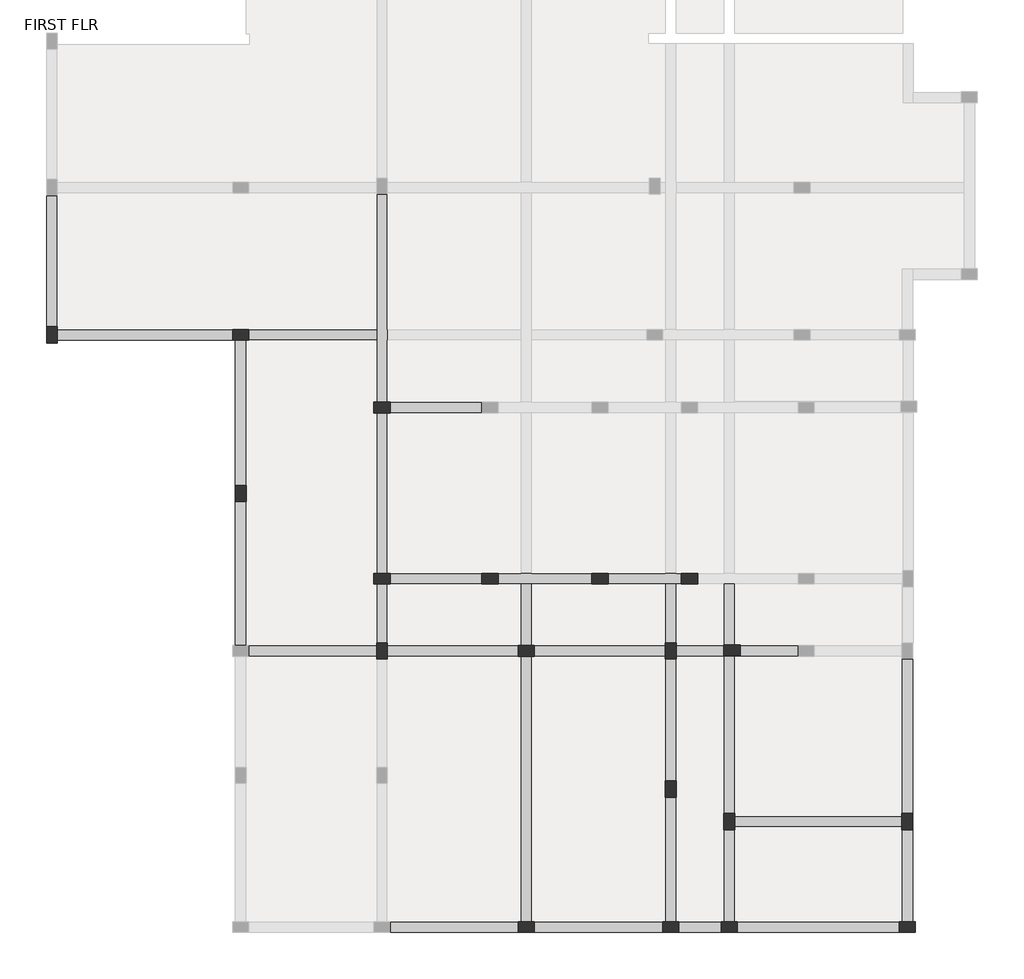
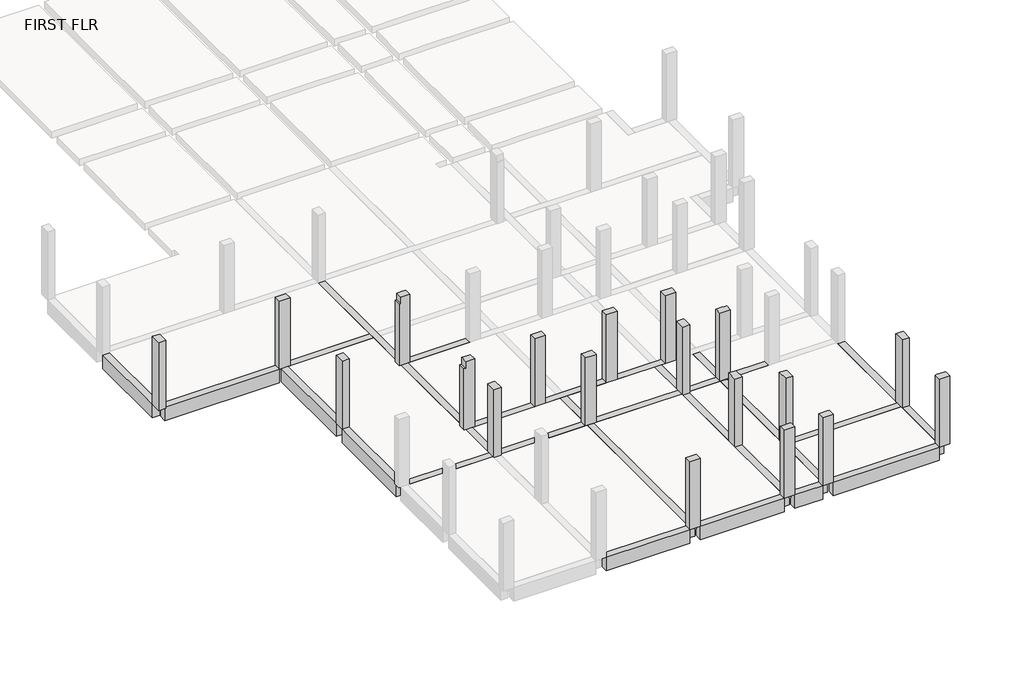
# One storey, part 2 of 5: 31 beams, 19 columns.
"""IFC4 building model written with IfcOpenShell, lengths in millimetres."""

from ifc_helpers import new_model, si_unit, frame, origin, place, context, project, spatial, polyline, outline, extrude, faceted_brep, element, save

model = new_model("IFC4")

# Units and contexts
model_context = context("Model", 3, world=origin())
ifc_project = project(units=[si_unit("LENGTHUNIT", "METRE", prefix="MILLI")], contexts=[model_context])

# Site, building, storey
site = spatial("IfcSite", under=ifc_project)
building = spatial("IfcBuilding", under=site)
storey = spatial("IfcBuildingStorey", under=building, Name="FIRST FLR", Elevation=3000.0)

# Beams
placement = place(None, origin())
element("IfcBeam", 1, ObjectType="M_Concrete-Rectangular Beam : 300 x 600mm", at=placement, inside=storey, context=model_context, shape_type="SweptSolid", body=[
    extrude(outline(polyline([(-10828.8105653, -2764.4535766), (-11128.8105653, -2764.4535766), (-11128.8105653, 876.1713929), (-10828.8105653, 876.1713929), (-10828.8105653, -2764.4535766)])), frame((0.0, 0.0, 2400.0), z_axis=(0.0, 0.0, 1.0), x_axis=(1.0, 0.0, 0.0)), (0.0, 0.0, 1.0), 600.0),
])
element("IfcBeam", 2, ObjectType="M_Concrete-Rectangular Beam : 300 x 600mm", at=placement, inside=storey, context=model_context, shape_type="Brep", body=[
    faceted_brep([(-5963.8105653, -3139.4535766, 3000.0), (-5963.8105653, -2839.4535766, 3000.0), (-10828.8105653, -2839.4535766, 3000.0), (-10828.8105653, -3139.4535766, 3000.0), (-5963.8105653, -3139.4535766, 2400.0), (-10828.8105653, -3139.4535766, 2400.0), (-5963.8105653, -2839.4535766, 2400.0), (-10828.8105653, -2839.4535766, 2400.0), (-5963.8105653, -2839.4535766, 2700.0), (-10828.8105653, -2839.4535766, 2700.0)], [[[0, 1, 2, 3]], [[4, 0, 3, 5]], [[6, 4, 5, 7]], [[2, 1, 8, 6, 7, 9]], [[1, 0, 4, 6, 8]], [[3, 2, 9, 7, 5]]]),
])
element("IfcBeam", 3, ObjectType="M_Concrete-Rectangular Beam : 300 x 600mm", at=placement, inside=storey, context=model_context, shape_type="Brep", body=[
    faceted_brep([(-5588.8105653, -7169.0760584, 3000.0), (-5588.8105653, -3139.4535766, 3000.0), (-5888.8105653, -3139.4535766, 3000.0), (-5888.8105653, -7169.0760584, 3000.0), (-5888.8105653, -3139.4535766, 2400.0), (-5888.8105653, -7169.0760584, 2400.0), (-5588.8105653, -3139.4535766, 2400.0), (-5588.8105653, -7169.0760584, 2400.0), (-5588.8105653, -7169.0760584, 2700.0), (-5588.8105653, -3139.4535766, 2700.0)], [[[0, 1, 2, 3]], [[3, 2, 4, 5]], [[5, 4, 6, 7]], [[1, 0, 8, 7, 6, 9]], [[6, 4, 2, 1, 9]], [[0, 3, 5, 7, 8]]]),
])
element("IfcBeam", 4, ObjectType="M_Concrete-Rectangular Beam : 300 x 600mm", at=placement, inside=storey, context=model_context, shape_type="Brep", body=[
    faceted_brep([(-5588.8105653, -11607.8970059, 3000.0), (-5588.8105653, -7619.0760584, 3000.0), (-5888.8105653, -7619.0760584, 3000.0), (-5888.8105653, -11607.8970059, 3000.0), (-5888.8105653, -7619.0760584, 2400.0), (-5888.8105653, -11607.8970059, 2400.0), (-5588.8105653, -7619.0760584, 2400.0), (-5588.8105653, -11607.8970059, 2400.0), (-5588.8105653, -11607.8970059, 2700.0), (-5588.8105653, -7619.0760584, 2700.0)], [[[0, 1, 2, 3]], [[3, 2, 4, 5]], [[5, 4, 6, 7]], [[1, 0, 8, 7, 6, 9]], [[0, 3, 5, 7, 8]], [[6, 4, 2, 1, 9]]]),
])
element("IfcBeam", 5, ObjectType="M_Concrete-Rectangular Beam : 300 x 600mm", at=placement, inside=storey, context=model_context, shape_type="SweptSolid", body=[
    extrude(outline(polyline([(1949.7296816, -19272.5304373), (1949.7296816, -19572.5304373), (-1596.7865686, -19572.5304373), (-1596.7865686, -19272.5304373), (1949.7296816, -19272.5304373)])), frame((0.0, 0.0, 2400.0), z_axis=(0.0, 0.0, 1.0), x_axis=(1.0, 0.0, 0.0)), (0.0, 0.0, 1.0), 600.0),
])
element("IfcBeam", 6, ObjectType="M_Concrete-Rectangular Beam : 300 x 600mm", at=placement, inside=storey, context=model_context, shape_type="SweptSolid", body=[
    extrude(outline(polyline([(5957.5248054, -19272.5304373), (5957.5248054, -19572.5304373), (2399.7296816, -19572.5304373), (2399.7296816, -19272.5304373), (5957.5248054, -19272.5304373)])), frame((0.0, 0.0, 2400.0), z_axis=(0.0, 0.0, 1.0), x_axis=(1.0, 0.0, 0.0)), (0.0, 0.0, 1.0), 600.0),
])
element("IfcBeam", 7, ObjectType="M_Concrete-Rectangular Beam : 300 x 600mm", at=placement, inside=storey, context=model_context, shape_type="SweptSolid", body=[
    extrude(outline(polyline([(7581.8679014, -19272.5304373), (7581.8679014, -19572.5304373), (6407.5248054, -19572.5304373), (6407.5248054, -19272.5304373), (7581.8679014, -19272.5304373)])), frame((0.0, 0.0, 2400.0), z_axis=(0.0, 0.0, 1.0), x_axis=(1.0, 0.0, 0.0)), (0.0, 0.0, 1.0), 600.0),
])
element("IfcBeam", 8, ObjectType="M_Concrete-Rectangular Beam : 300 x 600mm", at=placement, inside=storey, context=model_context, shape_type="SweptSolid", body=[
    extrude(outline(polyline([(12524.1163908, -19272.5304373), (12524.1163908, -19572.5304373), (8031.8679014, -19572.5304373), (8031.8679014, -19272.5304373), (12524.1163908, -19272.5304373)])), frame((0.0, 0.0, 2400.0), z_axis=(0.0, 0.0, 1.0), x_axis=(1.0, 0.0, 0.0)), (0.0, 0.0, 1.0), 600.0),
])
element("IfcBeam", 9, ObjectType="M_Concrete-Rectangular Beam : 300 x 600mm", at=placement, inside=storey, context=model_context, shape_type="Brep", body=[
    faceted_brep([(12599.1163908, -19272.5304373, 3000.0), (12899.1163908, -19272.5304373, 3000.0), (12899.1163908, -16719.1579597, 3000.0), (12599.1163908, -16719.1579597, 3000.0), (12899.1163908, -19272.5304373, 2400.0), (12899.1163908, -16719.1579597, 2400.0), (12599.1163908, -19272.5304373, 2400.0), (12599.1163908, -16719.1579597, 2400.0), (12599.1163908, -16719.1579597, 2700.0), (12599.1163908, -19272.5304373, 2700.0)], [[[0, 1, 2, 3]], [[1, 4, 5, 2]], [[4, 6, 7, 5]], [[0, 3, 8, 7, 6, 9]], [[6, 4, 1, 0, 9]], [[3, 2, 5, 7, 8]]]),
])
element("IfcBeam", 10, ObjectType="M_Concrete-Rectangular Beam : 300 x 600mm", at=placement, inside=storey, context=model_context, shape_type="Brep", body=[
    faceted_brep([(12599.1163908, -16269.1579597, 3000.0), (12899.1163908, -16269.1579597, 3000.0), (12899.1163908, -11982.8970059, 3000.0), (12599.1163908, -11982.8970059, 3000.0), (12899.1163908, -16269.1579597, 2400.0), (12899.1163908, -11982.8970059, 2400.0), (12599.1163908, -16269.1579597, 2400.0), (12599.1163908, -11982.8970059, 2400.0), (12599.1163908, -11982.8970059, 2700.0), (12599.1163908, -16269.1579597, 2700.0)], [[[0, 1, 2, 3]], [[1, 4, 5, 2]], [[4, 6, 7, 5]], [[0, 3, 8, 7, 6, 9]], [[6, 4, 1, 0, 9]], [[3, 2, 5, 7, 8]]]),
])
element("IfcBeam", 11, ObjectType="M_Concrete-Rectangular Beam : 300 x 600mm", at=placement, inside=storey, context=model_context, shape_type="Brep", body=[
    faceted_brep([(-1971.7865686, -9907.1078267, 3000.0), (-1971.7865686, -11532.8970059, 3000.0), (-1671.7865686, -11532.8970059, 3000.0), (-1671.7865686, -9907.1078267, 3000.0), (-1671.7865686, -11532.8970059, 2700.0), (-1671.7865686, -11532.8970059, 2400.0), (-1671.7865686, -9907.1078267, 2400.0), (-1671.7865686, -9907.1078267, 2700.0), (-1971.7865686, -11532.8970059, 2400.0), (-1971.7865686, -9907.1078267, 2400.0), (-1971.7865686, -9907.1078267, 2700.0), (-1971.7865686, -11532.8970059, 2700.0)], [[[0, 1, 2, 3]], [[3, 2, 4, 5, 6, 7]], [[6, 5, 8, 9]], [[1, 0, 10, 9, 8, 11]], [[0, 3, 7, 6, 9, 10]], [[8, 5, 4, 2, 1, 11]]]),
])
element("IfcBeam", 12, ObjectType="M_Concrete-Rectangular Beam : 300 x 600mm", at=placement, inside=storey, context=model_context, shape_type="Brep", body=[
    faceted_brep([(-1671.7865686, 916.1713929, 3000.0), (-1971.7865686, 916.1713929, 3000.0), (-1971.7865686, -2839.4535766, 3000.0), (-1971.7865686, -3139.4535766, 3000.0), (-1971.7865686, -4851.6229916, 3000.0), (-1671.7865686, -4851.6229916, 3000.0), (-1671.7865686, -3139.4535766, 3000.0), (-1671.7865686, -2839.4535766, 3000.0), (-1971.7865686, 916.1713929, 2400.0), (-1971.7865686, -2839.4535766, 2400.0), (-1971.7865686, -3139.4535766, 2400.0), (-1971.7865686, -4851.6229916, 2400.0), (-1971.7865686, -4851.6229916, 2700.0), (-1971.7865686, 916.1713929, 2700.0), (-1671.7865686, 916.1713929, 2400.0), (-1671.7865686, -2839.4535766, 2400.0), (-1671.7865686, -3139.4535766, 2400.0), (-1671.7865686, -4851.6229916, 2400.0), (-1671.7865686, 916.1713929, 2700.0), (-1671.7865686, -4851.6229916, 2700.0)], [[[0, 1, 2, 3, 4, 5, 6, 7]], [[8, 9, 10, 11, 12, 4, 3, 2, 1, 13]], [[8, 14, 15, 16, 17, 11, 10, 9]], [[17, 16, 15, 14, 18, 0, 7, 6, 5, 19]], [[1, 0, 18, 14, 8, 13]], [[5, 4, 12, 11, 17, 19]]]),
])
element("IfcBeam", 13, ObjectType="M_Concrete-Rectangular Beam : 300 x 600mm", at=placement, inside=storey, context=model_context, shape_type="Brep", body=[
    faceted_brep([(-1671.7865686, -5151.6229916, 3000.0), (-1971.7865686, -5151.6229916, 3000.0), (-1971.7865686, -9607.1078267, 3000.0), (-1671.7865686, -9607.1078267, 3000.0), (-1971.7865686, -5151.6229916, 2700.0), (-1971.7865686, -5151.6229916, 2400.0), (-1971.7865686, -9607.1078267, 2400.0), (-1971.7865686, -9607.1078267, 2700.0), (-1671.7865686, -5151.6229916, 2400.0), (-1671.7865686, -9607.1078267, 2400.0), (-1671.7865686, -9607.1078267, 2700.0), (-1671.7865686, -5151.6229916, 2700.0)], [[[0, 1, 2, 3]], [[2, 1, 4, 5, 6, 7]], [[5, 8, 9, 6]], [[0, 3, 10, 9, 8, 11]], [[1, 0, 11, 8, 5, 4]], [[3, 2, 7, 6, 9, 10]]]),
])
element("IfcBeam", 14, ObjectType="M_Concrete-Rectangular Beam : 300 x 600mm", at=placement, inside=storey, context=model_context, shape_type="Brep", body=[
    faceted_brep([(2324.7296816, -11907.8970059, 3000.0), (2024.7296816, -11907.8970059, 3000.0), (2024.7296816, -19272.5304373, 3000.0), (2324.7296816, -19272.5304373, 3000.0), (2024.7296816, -11907.8970059, 2700.0), (2024.7296816, -11907.8970059, 2400.0), (2024.7296816, -19272.5304373, 2400.0), (2024.7296816, -19272.5304373, 2700.0), (2324.7296816, -11907.8970059, 2400.0), (2324.7296816, -19272.5304373, 2400.0), (2324.7296816, -19272.5304373, 2700.0), (2324.7296816, -11907.8970059, 2700.0)], [[[0, 1, 2, 3]], [[2, 1, 4, 5, 6, 7]], [[5, 8, 9, 6]], [[0, 3, 10, 9, 8, 11]], [[1, 0, 11, 8, 5, 4]], [[3, 2, 7, 6, 9, 10]]]),
])
element("IfcBeam", 15, ObjectType="M_Concrete-Rectangular Beam : 300 x 600mm", at=placement, inside=storey, context=model_context, shape_type="Brep", body=[
    faceted_brep([(6332.5248054, -11982.8970059, 3000.0), (6032.5248054, -11982.8970059, 3000.0), (6032.5248054, -15369.1579597, 3000.0), (6332.5248054, -15369.1579597, 3000.0), (6032.5248054, -11982.8970059, 2700.0), (6032.5248054, -11982.8970059, 2400.0), (6032.5248054, -15369.1579597, 2400.0), (6032.5248054, -15369.1579597, 2700.0), (6332.5248054, -11982.8970059, 2400.0), (6332.5248054, -15369.1579597, 2400.0), (6332.5248054, -15369.1579597, 2700.0), (6332.5248054, -11982.8970059, 2700.0)], [[[0, 1, 2, 3]], [[2, 1, 4, 5, 6, 7]], [[5, 8, 9, 6]], [[0, 3, 10, 9, 8, 11]], [[1, 0, 11, 8, 5, 4]], [[3, 2, 7, 6, 9, 10]]]),
])
element("IfcBeam", 16, ObjectType="M_Concrete-Rectangular Beam : 300 x 600mm", at=placement, inside=storey, context=model_context, shape_type="Brep", body=[
    faceted_brep([(6032.5248054, -19272.5304373, 3000.0), (6332.5248054, -19272.5304373, 3000.0), (6332.5248054, -15819.1579597, 3000.0), (6032.5248054, -15819.1579597, 3000.0), (6032.5248054, -15819.1579597, 2700.0), (6032.5248054, -15819.1579597, 2400.0), (6032.5248054, -19272.5304373, 2400.0), (6032.5248054, -19272.5304373, 2700.0), (6332.5248054, -19272.5304373, 2400.0), (6332.5248054, -15819.1579597, 2400.0), (6332.5248054, -19272.5304373, 2700.0), (6332.5248054, -15819.1579597, 2700.0)], [[[0, 1, 2, 3]], [[0, 3, 4, 5, 6, 7]], [[8, 6, 5, 9]], [[2, 1, 10, 8, 9, 11]], [[1, 0, 7, 6, 8, 10]], [[3, 2, 11, 9, 5, 4]]]),
])
element("IfcBeam", 17, ObjectType="M_Concrete-Rectangular Beam : 300 x 600mm", at=placement, inside=storey, context=model_context, shape_type="Brep", body=[
    faceted_brep([(7656.8679014, -19272.5304373, 3000.0), (7956.8679014, -19272.5304373, 3000.0), (7956.8679014, -16719.1579597, 3000.0), (7656.8679014, -16719.1579597, 3000.0), (7656.8679014, -16719.1579597, 2700.0), (7656.8679014, -16719.1579597, 2400.0), (7656.8679014, -19272.5304373, 2400.0), (7656.8679014, -19272.5304373, 2700.0), (7956.8679014, -19272.5304373, 2400.0), (7956.8679014, -16719.1579597, 2400.0), (7956.8679014, -19272.5304373, 2700.0), (7956.8679014, -16719.1579597, 2700.0)], [[[0, 1, 2, 3]], [[0, 3, 4, 5, 6, 7]], [[8, 6, 5, 9]], [[2, 1, 10, 8, 9, 11]], [[1, 0, 7, 6, 8, 10]], [[3, 2, 11, 9, 5, 4]]]),
])
element("IfcBeam", 18, ObjectType="M_Concrete-Rectangular Beam : 300 x 600mm", at=placement, inside=storey, context=model_context, shape_type="Brep", body=[
    faceted_brep([(-5513.8105653, -2839.4535766, 3000.0), (-5513.8105653, -3139.4535766, 3000.0), (-1971.7865686, -3139.4535766, 3000.0), (-1971.7865686, -2839.4535766, 3000.0), (-5513.8105653, -3139.4535766, 2700.0), (-5513.8105653, -3139.4535766, 2400.0), (-1971.7865686, -3139.4535766, 2400.0), (-1971.7865686, -3139.4535766, 2700.0), (-5513.8105653, -2839.4535766, 2400.0), (-1971.7865686, -2839.4535766, 2400.0), (-1971.7865686, -2839.4535766, 2700.0), (-5513.8105653, -2839.4535766, 2700.0)], [[[0, 1, 2, 3]], [[2, 1, 4, 5, 6, 7]], [[5, 8, 9, 6]], [[0, 3, 10, 9, 8, 11]], [[1, 0, 11, 8, 5, 4]], [[3, 2, 7, 6, 9, 10]]]),
])
element("IfcBeam", 19, ObjectType="M_Concrete-Rectangular Beam : 300 x 600mm", at=placement, inside=storey, context=model_context, shape_type="Brep", body=[
    faceted_brep([(-1596.7865686, -4851.6229916, 3000.0), (-1596.7865686, -5151.6229916, 3000.0), (949.7296816, -5151.6229916, 3000.0), (949.7296816, -4851.6229916, 3000.0), (-1596.7865686, -5151.6229916, 2700.0), (-1596.7865686, -5151.6229916, 2400.0), (949.7296816, -5151.6229916, 2400.0), (949.7296816, -5151.6229916, 2700.0), (-1596.7865686, -4851.6229916, 2400.0), (949.7296816, -4851.6229916, 2400.0), (949.7296816, -4851.6229916, 2700.0), (-1596.7865686, -4851.6229916, 2700.0)], [[[0, 1, 2, 3]], [[2, 1, 4, 5, 6, 7]], [[5, 8, 9, 6]], [[0, 3, 10, 9, 8, 11]], [[1, 0, 11, 8, 5, 4]], [[3, 2, 7, 6, 9, 10]]]),
])
element("IfcBeam", 20, ObjectType="M_Concrete-Rectangular Beam : 300 x 600mm", at=placement, inside=storey, context=model_context, shape_type="Brep", body=[
    faceted_brep([(-1971.7865686, -11907.8970059, 3000.0), (-1971.7865686, -11607.8970059, 3000.0), (-5513.8105653, -11607.8970059, 3000.0), (-5513.8105653, -11907.8970059, 3000.0), (-5513.8105653, -11907.8970059, 2700.0), (-5513.8105653, -11907.8970059, 2400.0), (-1971.7865686, -11907.8970059, 2400.0), (-1971.7865686, -11907.8970059, 2700.0), (-1971.7865686, -11607.8970059, 2400.0), (-5513.8105653, -11607.8970059, 2400.0), (-1971.7865686, -11607.8970059, 2700.0), (-5513.8105653, -11607.8970059, 2700.0)], [[[0, 1, 2, 3]], [[0, 3, 4, 5, 6, 7]], [[8, 6, 5, 9]], [[2, 1, 10, 8, 9, 11]], [[1, 0, 7, 6, 8, 10]], [[3, 2, 11, 9, 5, 4]]]),
])
element("IfcBeam", 21, ObjectType="M_Concrete-Rectangular Beam : 300 x 600mm", at=placement, inside=storey, context=model_context, shape_type="Brep", body=[
    faceted_brep([(1949.7296816, -11907.8970059, 3000.0), (1949.7296816, -11607.8970059, 3000.0), (-1671.7865686, -11607.8970059, 3000.0), (-1671.7865686, -11907.8970059, 3000.0), (-1671.7865686, -11907.8970059, 2700.0), (-1671.7865686, -11907.8970059, 2400.0), (1949.7296816, -11907.8970059, 2400.0), (1949.7296816, -11907.8970059, 2700.0), (1949.7296816, -11607.8970059, 2400.0), (-1671.7865686, -11607.8970059, 2400.0), (1949.7296816, -11607.8970059, 2700.0), (-1671.7865686, -11607.8970059, 2700.0)], [[[0, 1, 2, 3]], [[0, 3, 4, 5, 6, 7]], [[8, 6, 5, 9]], [[2, 1, 10, 8, 9, 11]], [[1, 0, 7, 6, 8, 10]], [[3, 2, 11, 9, 5, 4]]]),
])
element("IfcBeam", 22, ObjectType="M_Concrete-Rectangular Beam : 300 x 600mm", at=placement, inside=storey, context=model_context, shape_type="Brep", body=[
    faceted_brep([(6032.5248054, -11907.8970059, 3000.0), (6032.5248054, -11607.8970059, 3000.0), (2399.7296816, -11607.8970059, 3000.0), (2399.7296816, -11907.8970059, 3000.0), (2399.7296816, -11907.8970059, 2700.0), (2399.7296816, -11907.8970059, 2400.0), (6032.5248054, -11907.8970059, 2400.0), (6032.5248054, -11907.8970059, 2700.0), (6032.5248054, -11607.8970059, 2400.0), (2399.7296816, -11607.8970059, 2400.0), (6032.5248054, -11607.8970059, 2700.0), (2399.7296816, -11607.8970059, 2700.0)], [[[0, 1, 2, 3]], [[0, 3, 4, 5, 6, 7]], [[8, 6, 5, 9]], [[2, 1, 10, 8, 9, 11]], [[1, 0, 7, 6, 8, 10]], [[3, 2, 11, 9, 5, 4]]]),
])
element("IfcBeam", 23, ObjectType="M_Concrete-Rectangular Beam : 300 x 600mm", at=placement, inside=storey, context=model_context, shape_type="Brep", body=[
    faceted_brep([(9721.8679014, -11907.8970059, 3000.0), (9721.8679014, -11607.8970059, 3000.0), (8111.8679014, -11607.8970059, 3000.0), (8111.8679014, -11887.8970059, 3000.0), (7661.8679014, -11887.8970059, 3000.0), (7661.8679014, -11607.8970059, 3000.0), (7656.8679014, -11607.8970059, 3000.0), (6332.5248054, -11607.8970059, 3000.0), (6332.5248054, -11907.8970059, 3000.0), (7656.8679014, -11907.8970059, 3000.0), (7956.8679014, -11907.8970059, 3000.0), (6332.5248054, -11907.8970059, 2400.0), (7656.8679014, -11907.8970059, 2400.0), (7956.8679014, -11907.8970059, 2400.0), (9721.8679014, -11907.8970059, 2400.0), (9721.8679014, -11907.8970059, 2700.0), (6332.5248054, -11907.8970059, 2700.0), (9721.8679014, -11607.8970059, 2400.0), (6332.5248054, -11607.8970059, 2400.0), (7656.8679014, -11607.8970059, 2400.0), (7661.8679014, -11607.8970059, 2400.0), (7661.8679014, -11887.8970059, 2400.0), (8111.8679014, -11887.8970059, 2400.0), (8111.8679014, -11607.8970059, 2400.0), (6332.5248054, -11607.8970059, 2700.0), (9721.8679014, -11607.8970059, 2700.0), (8111.8679014, -11607.8970059, 2700.0)], [[[0, 1, 2, 3, 4, 5, 6, 7, 8, 9, 10]], [[11, 12, 13, 14, 15, 0, 10, 9, 8, 16]], [[17, 14, 13, 12, 11, 18, 19, 20, 21, 22, 23]], [[20, 19, 18, 24, 7, 6, 5]], [[1, 0, 15, 14, 17, 25]], [[8, 7, 24, 18, 11, 16]], [[22, 3, 2, 26, 23]], [[3, 22, 21, 4]], [[4, 21, 20, 5]], [[2, 1, 25, 17, 23, 26]]]),
])
element("IfcBeam", 24, ObjectType="M_Concrete-Rectangular Beam : 300 x 600mm", at=placement, inside=storey, context=model_context, shape_type="Brep", body=[
    faceted_brep([(12599.1163908, -16644.1579597, 3000.0), (12599.1163908, -16344.1579597, 3000.0), (7956.8679014, -16344.1579597, 3000.0), (7956.8679014, -16644.1579597, 3000.0), (7956.8679014, -16644.1579597, 2700.0), (7956.8679014, -16644.1579597, 2400.0), (12599.1163908, -16644.1579597, 2400.0), (12599.1163908, -16644.1579597, 2700.0), (12599.1163908, -16344.1579597, 2400.0), (7956.8679014, -16344.1579597, 2400.0), (12599.1163908, -16344.1579597, 2700.0), (7956.8679014, -16344.1579597, 2700.0)], [[[0, 1, 2, 3]], [[0, 3, 4, 5, 6, 7]], [[8, 6, 5, 9]], [[2, 1, 10, 8, 9, 11]], [[1, 0, 7, 6, 8, 10]], [[3, 2, 11, 9, 5, 4]]]),
])
element("IfcBeam", 25, ObjectType="M_Concrete-Rectangular Beam : 300 x 600mm", at=placement, inside=storey, context=model_context, shape_type="Brep", body=[
    faceted_brep([(-1596.7865686, -9607.1078267, 3000.0), (-1596.7865686, -9907.1078267, 3000.0), (949.7296816, -9907.1078267, 3000.0), (949.7296816, -9607.1078267, 3000.0), (-1596.7865686, -9907.1078267, 2700.0), (-1596.7865686, -9907.1078267, 2400.0), (949.7296816, -9907.1078267, 2400.0), (949.7296816, -9907.1078267, 2700.0), (-1596.7865686, -9607.1078267, 2400.0), (949.7296816, -9607.1078267, 2400.0), (949.7296816, -9607.1078267, 2700.0), (-1596.7865686, -9607.1078267, 2700.0)], [[[0, 1, 2, 3]], [[2, 1, 4, 5, 6, 7]], [[5, 8, 9, 6]], [[0, 3, 10, 9, 8, 11]], [[1, 0, 11, 8, 5, 4]], [[3, 2, 7, 6, 9, 10]]]),
])
element("IfcBeam", 26, ObjectType="M_Concrete-Rectangular Beam : 300 x 600mm", at=placement, inside=storey, context=model_context, shape_type="Brep", body=[
    faceted_brep([(1399.7296816, -9607.1078267, 3000.0), (1399.7296816, -9907.1078267, 3000.0), (2024.7296816, -9907.1078267, 3000.0), (2324.7296816, -9907.1078267, 3000.0), (3997.5248054, -9907.1078267, 3000.0), (3997.5248054, -9607.1078267, 3000.0), (2324.7296816, -9607.1078267, 3000.0), (2024.7296816, -9607.1078267, 3000.0), (1399.7296816, -9907.1078267, 2400.0), (2024.7296816, -9907.1078267, 2400.0), (2324.7296816, -9907.1078267, 2400.0), (3997.5248054, -9907.1078267, 2400.0), (3997.5248054, -9907.1078267, 2700.0), (1399.7296816, -9907.1078267, 2700.0), (1399.7296816, -9607.1078267, 2400.0), (2024.7296816, -9607.1078267, 2400.0), (2324.7296816, -9607.1078267, 2400.0), (3997.5248054, -9607.1078267, 2400.0), (1399.7296816, -9607.1078267, 2700.0), (3997.5248054, -9607.1078267, 2700.0)], [[[0, 1, 2, 3, 4, 5, 6, 7]], [[8, 9, 10, 11, 12, 4, 3, 2, 1, 13]], [[8, 14, 15, 16, 17, 11, 10, 9]], [[17, 16, 15, 14, 18, 0, 7, 6, 5, 19]], [[1, 0, 18, 14, 8, 13]], [[5, 4, 12, 11, 17, 19]]]),
])
element("IfcBeam", 27, ObjectType="M_Concrete-Rectangular Beam : 300 x 600mm", at=placement, inside=storey, context=model_context, shape_type="Brep", body=[
    faceted_brep([(4447.5248054, -9607.1078267, 3000.0), (4447.5248054, -9907.1078267, 3000.0), (6032.5248054, -9907.1078267, 3000.0), (6332.5248054, -9907.1078267, 3000.0), (6481.8679014, -9907.1078267, 3000.0), (6481.8679014, -9607.1078267, 3000.0), (6332.5248054, -9607.1078267, 3000.0), (6032.5248054, -9607.1078267, 3000.0), (4447.5248054, -9907.1078267, 2400.0), (6032.5248054, -9907.1078267, 2400.0), (6332.5248054, -9907.1078267, 2400.0), (6481.8679014, -9907.1078267, 2400.0), (6481.8679014, -9907.1078267, 2700.0), (4447.5248054, -9907.1078267, 2700.0), (4447.5248054, -9607.1078267, 2400.0), (6032.5248054, -9607.1078267, 2400.0), (6332.5248054, -9607.1078267, 2400.0), (6481.8679014, -9607.1078267, 2400.0), (4447.5248054, -9607.1078267, 2700.0), (6481.8679014, -9607.1078267, 2700.0)], [[[0, 1, 2, 3, 4, 5, 6, 7]], [[8, 9, 10, 11, 12, 4, 3, 2, 1, 13]], [[8, 14, 15, 16, 17, 11, 10, 9]], [[17, 16, 15, 14, 18, 0, 7, 6, 5, 19]], [[1, 0, 18, 14, 8, 13]], [[5, 4, 12, 11, 17, 19]]]),
])
element("IfcBeam", 28, ObjectType="M_Concrete-Rectangular Beam : 300 x 600mm", at=placement, inside=storey, context=model_context, shape_type="Brep", body=[
    faceted_brep([(7656.8679014, -16269.1579597, 3000.0), (7956.8679014, -16269.1579597, 3000.0), (7956.8679014, -11907.8970059, 3000.0), (7656.8679014, -11907.8970059, 3000.0), (7656.8679014, -11907.8970059, 2700.0), (7656.8679014, -11907.8970059, 2400.0), (7656.8679014, -16269.1579597, 2400.0), (7656.8679014, -16269.1579597, 2700.0), (7956.8679014, -16269.1579597, 2400.0), (7956.8679014, -11907.8970059, 2400.0), (7956.8679014, -16269.1579597, 2700.0), (7956.8679014, -11907.8970059, 2700.0)], [[[0, 1, 2, 3]], [[0, 3, 4, 5, 6, 7]], [[8, 6, 5, 9]], [[2, 1, 10, 8, 9, 11]], [[1, 0, 7, 6, 8, 10]], [[3, 2, 11, 9, 5, 4]]]),
])
element("IfcBeam", 29, ObjectType="M_Concrete-Rectangular Beam : 300 x 600mm", at=placement, inside=storey, context=model_context, shape_type="Brep", body=[
    faceted_brep([(2024.7296816, -11607.8970059, 3000.0), (2324.7296816, -11607.8970059, 3000.0), (2324.7296816, -9907.1078267, 3000.0), (2024.7296816, -9907.1078267, 3000.0), (2024.7296816, -9907.1078267, 2700.0), (2024.7296816, -9907.1078267, 2400.0), (2024.7296816, -11607.8970059, 2400.0), (2024.7296816, -11607.8970059, 2700.0), (2324.7296816, -11607.8970059, 2400.0), (2324.7296816, -9907.1078267, 2400.0), (2324.7296816, -11607.8970059, 2700.0), (2324.7296816, -9907.1078267, 2700.0)], [[[0, 1, 2, 3]], [[0, 3, 4, 5, 6, 7]], [[8, 6, 5, 9]], [[2, 1, 10, 8, 9, 11]], [[1, 0, 7, 6, 8, 10]], [[3, 2, 11, 9, 5, 4]]]),
])
element("IfcBeam", 30, ObjectType="M_Concrete-Rectangular Beam : 300 x 600mm", at=placement, inside=storey, context=model_context, shape_type="Brep", body=[
    faceted_brep([(6032.5248054, -11532.8970059, 3000.0), (6332.5248054, -11532.8970059, 3000.0), (6332.5248054, -9907.1078267, 3000.0), (6032.5248054, -9907.1078267, 3000.0), (6032.5248054, -9907.1078267, 2700.0), (6032.5248054, -9907.1078267, 2400.0), (6032.5248054, -11532.8970059, 2400.0), (6032.5248054, -11532.8970059, 2700.0), (6332.5248054, -11532.8970059, 2400.0), (6332.5248054, -9907.1078267, 2400.0), (6332.5248054, -11532.8970059, 2700.0), (6332.5248054, -9907.1078267, 2700.0)], [[[0, 1, 2, 3]], [[0, 3, 4, 5, 6, 7]], [[8, 6, 5, 9]], [[2, 1, 10, 8, 9, 11]], [[1, 0, 7, 6, 8, 10]], [[3, 2, 11, 9, 5, 4]]]),
])
element("IfcBeam", 31, ObjectType="M_Concrete-Rectangular Beam : 300 x 600mm", at=placement, inside=storey, context=model_context, shape_type="Brep", body=[
    faceted_brep([(7661.8679014, -11587.8970059, 3000.0), (7956.8679014, -11587.8970059, 3000.0), (7956.8679014, -9907.1078267, 3000.0), (7656.8679014, -9907.1078267, 3000.0), (7656.8679014, -11607.8970059, 3000.0), (7661.8679014, -11607.8970059, 3000.0), (7656.8679014, -9907.1078267, 2700.0), (7656.8679014, -9907.1078267, 2400.0), (7656.8679014, -11607.8970059, 2400.0), (7656.8679014, -11607.8970059, 2700.0), (7956.8679014, -11587.8970059, 2400.0), (7661.8679014, -11587.8970059, 2400.0), (7661.8679014, -11607.8970059, 2400.0), (7956.8679014, -9907.1078267, 2400.0), (7956.8679014, -11587.8970059, 2700.0), (7956.8679014, -9907.1078267, 2700.0)], [[[0, 1, 2, 3, 4, 5]], [[4, 3, 6, 7, 8, 9]], [[10, 11, 12, 8, 7, 13]], [[2, 1, 14, 10, 13, 15]], [[0, 11, 10, 14, 1]], [[11, 0, 5, 12]], [[3, 2, 15, 13, 7, 6]], [[5, 4, 9, 8, 12]]]),
])

# Columns
element("IfcColumn", 32, ObjectType="M_Concrete-Rectangular-Column : 300 x 450mm", at=placement, inside=storey, context=model_context, shape_type="Brep", body=[
    faceted_brep([(-11128.8105653, -3214.4535766, 3000.0), (-11128.8105653, -2764.4535766, 3000.0), (-10828.8105653, -2764.4535766, 3000.0), (-10828.8105653, -3214.4535766, 3000.0), (-11128.8105653, -3214.4535766, 6048.0), (-11128.8105653, -2764.4535766, 6048.0), (-10828.8105653, -2764.4535766, 6048.0), (-10828.8105653, -2839.4535766, 6048.0), (-10828.8105653, -3214.4535766, 6048.0)], [[[0, 1, 2, 3]], [[4, 5, 1, 0]], [[5, 6, 2, 1]], [[6, 7, 8, 3, 2]], [[8, 4, 0, 3]], [[4, 8, 7, 6, 5]]]),
])
element("IfcColumn", 33, ObjectType="M_Concrete-Rectangular-Column : 300 x 450mm", at=placement, inside=storey, context=model_context, shape_type="Brep", body=[
    faceted_brep([(-5513.8105653, -3139.4535766, 3000.0), (-5963.8105653, -3139.4535766, 3000.0), (-5963.8105653, -2839.4535766, 3000.0), (-5513.8105653, -2839.4535766, 3000.0), (-5513.8105653, -3139.4535766, 5748.0), (-5513.8105653, -3139.4535766, 6048.0), (-5588.8105653, -3139.4535766, 6048.0), (-5963.8105653, -3139.4535766, 6048.0), (-5963.8105653, -2839.4535766, 6048.0), (-5963.8105653, -2839.4535766, 5748.0), (-5513.8105653, -2839.4535766, 6048.0), (-5513.8105653, -2839.4535766, 5748.0)], [[[0, 1, 2, 3]], [[1, 0, 4, 5, 6, 7]], [[2, 1, 7, 8, 9]], [[3, 2, 9, 8, 10, 11]], [[0, 3, 11, 10, 5, 4]], [[8, 7, 6, 5, 10]]]),
])
element("IfcColumn", 34, ObjectType="M_Concrete-Rectangular-Column : 300 x 450mm", at=placement, inside=storey, context=model_context, shape_type="Brep", body=[
    faceted_brep([(-1596.7865686, -5151.6229916, 3000.0), (-2046.7865686, -5151.6229916, 3000.0), (-2046.7865686, -4851.6229916, 3000.0), (-1596.7865686, -4851.6229916, 3000.0), (-1596.7865686, -5151.6229916, 5748.0), (-1596.7865686, -5151.6229916, 6048.0), (-1671.7865686, -5151.6229916, 6048.0), (-1971.7865686, -5151.6229916, 6048.0), (-1971.7865686, -5151.6229916, 5748.0), (-2046.7865686, -5151.6229916, 5748.0), (-2046.7865686, -4851.6229916, 5748.0), (-1971.7865686, -4851.6229916, 5748.0), (-1971.7865686, -4851.6229916, 6048.0), (-1671.7865686, -4851.6229916, 6048.0), (-1596.7865686, -4851.6229916, 6048.0), (-1596.7865686, -4851.6229916, 5748.0)], [[[0, 1, 2, 3]], [[1, 0, 4, 5, 6, 7, 8, 9]], [[2, 1, 9, 10]], [[3, 2, 10, 11, 12, 13, 14, 15]], [[0, 3, 15, 14, 5, 4]], [[5, 14, 13, 12, 7, 6]], [[8, 11, 10, 9]], [[11, 8, 7, 12]]]),
])
element("IfcColumn", 35, ObjectType="M_Concrete-Rectangular-Column : 300 x 450mm", at=placement, inside=storey, context=model_context, shape_type="Brep", body=[
    faceted_brep([(-1596.7865686, -9907.1078267, 3000.0), (-2046.7865686, -9907.1078267, 3000.0), (-2046.7865686, -9607.1078267, 3000.0), (-1596.7865686, -9607.1078267, 3000.0), (-1596.7865686, -9907.1078267, 5748.0), (-1596.7865686, -9907.1078267, 6048.0), (-1671.7865686, -9907.1078267, 6048.0), (-1971.7865686, -9907.1078267, 6048.0), (-1971.7865686, -9907.1078267, 5748.0), (-2046.7865686, -9907.1078267, 5748.0), (-2046.7865686, -9607.1078267, 5748.0), (-1971.7865686, -9607.1078267, 5748.0), (-1971.7865686, -9607.1078267, 6048.0), (-1671.7865686, -9607.1078267, 6048.0), (-1596.7865686, -9607.1078267, 6048.0), (-1596.7865686, -9607.1078267, 5748.0)], [[[0, 1, 2, 3]], [[1, 0, 4, 5, 6, 7, 8, 9]], [[2, 1, 9, 10]], [[3, 2, 10, 11, 12, 13, 14, 15]], [[0, 3, 15, 14, 5, 4]], [[5, 14, 13, 12, 7, 6]], [[8, 11, 10, 9]], [[11, 8, 7, 12]]]),
])
element("IfcColumn", 36, ObjectType="M_Concrete-Rectangular-Column : 300 x 450mm", at=placement, inside=storey, context=model_context, shape_type="Brep", body=[
    faceted_brep([(1399.7296816, -9907.1078267, 3000.0), (949.7296816, -9907.1078267, 3000.0), (949.7296816, -9607.1078267, 3000.0), (1399.7296816, -9607.1078267, 3000.0), (1399.7296816, -9907.1078267, 5748.0), (1399.7296816, -9907.1078267, 6048.0), (949.7296816, -9907.1078267, 6048.0), (949.7296816, -9907.1078267, 5748.0), (949.7296816, -9607.1078267, 6048.0), (949.7296816, -9607.1078267, 5748.0), (1399.7296816, -9607.1078267, 6048.0), (1399.7296816, -9607.1078267, 5748.0)], [[[0, 1, 2, 3]], [[1, 0, 4, 5, 6, 7]], [[2, 1, 7, 6, 8, 9]], [[3, 2, 9, 8, 10, 11]], [[0, 3, 11, 10, 5, 4]], [[6, 5, 10, 8]]]),
])
element("IfcColumn", 37, ObjectType="M_Concrete-Rectangular-Column : 300 x 450mm", at=placement, inside=storey, context=model_context, shape_type="Brep", body=[
    faceted_brep([(4447.5248054, -9907.1078267, 3000.0), (3997.5248054, -9907.1078267, 3000.0), (3997.5248054, -9607.1078267, 3000.0), (4447.5248054, -9607.1078267, 3000.0), (4447.5248054, -9907.1078267, 5748.0), (4447.5248054, -9907.1078267, 6048.0), (3997.5248054, -9907.1078267, 6048.0), (3997.5248054, -9907.1078267, 5748.0), (3997.5248054, -9607.1078267, 6048.0), (3997.5248054, -9607.1078267, 5748.0), (4447.5248054, -9607.1078267, 6048.0), (4447.5248054, -9607.1078267, 5748.0)], [[[0, 1, 2, 3]], [[1, 0, 4, 5, 6, 7]], [[2, 1, 7, 6, 8, 9]], [[3, 2, 9, 8, 10, 11]], [[0, 3, 11, 10, 5, 4]], [[6, 5, 10, 8]]]),
])
element("IfcColumn", 38, ObjectType="M_Concrete-Rectangular-Column : 300 x 450mm", at=placement, inside=storey, context=model_context, shape_type="Brep", body=[
    faceted_brep([(6931.8679014, -9907.1078267, 3000.0), (6481.8679014, -9907.1078267, 3000.0), (6481.8679014, -9607.1078267, 3000.0), (6931.8679014, -9607.1078267, 3000.0), (6931.8679014, -9907.1078267, 5748.0), (6931.8679014, -9907.1078267, 6048.0), (6481.8679014, -9907.1078267, 6048.0), (6481.8679014, -9907.1078267, 5748.0), (6481.8679014, -9607.1078267, 6048.0), (6481.8679014, -9607.1078267, 5748.0), (6931.8679014, -9607.1078267, 6048.0), (6931.8679014, -9607.1078267, 5748.0)], [[[0, 1, 2, 3]], [[1, 0, 4, 5, 6, 7]], [[2, 1, 7, 6, 8, 9]], [[3, 2, 9, 8, 10, 11]], [[0, 3, 11, 10, 5, 4]], [[6, 5, 10, 8]]]),
])
element("IfcColumn", 39, ObjectType="M_Concrete-Rectangular-Column : 300 x 450mm", at=placement, inside=storey, context=model_context, shape_type="Brep", body=[
    faceted_brep([(7661.8679014, -11587.8970059, 3000.0), (8111.8679014, -11587.8970059, 3000.0), (8111.8679014, -11887.8970059, 3000.0), (7661.8679014, -11887.8970059, 3000.0), (7661.8679014, -11587.8970059, 6048.0), (7956.8679014, -11587.8970059, 6048.0), (7956.8679014, -11587.8970059, 5748.0), (8111.8679014, -11587.8970059, 5748.0), (8111.8679014, -11607.8970059, 5748.0), (8111.8679014, -11607.8970059, 6048.0), (8111.8679014, -11887.8970059, 6048.0), (8111.8679014, -11887.8970059, 5448.0), (7661.8679014, -11887.8970059, 6048.0), (7661.8679014, -11887.8970059, 5448.0), (7661.8679014, -11607.8970059, 6048.0), (7956.8679014, -11607.8970059, 6048.0), (7956.8679014, -11607.8970059, 5748.0)], [[[0, 1, 2, 3]], [[1, 0, 4, 5, 6, 7]], [[2, 1, 7, 8, 9, 10, 11]], [[3, 2, 11, 10, 12, 13]], [[0, 3, 13, 12, 14, 4]], [[12, 10, 9, 15, 5, 4, 14]], [[6, 16, 8, 7]], [[16, 15, 9, 8]], [[15, 16, 6, 5]]]),
])
element("IfcColumn", 40, ObjectType="M_Concrete-Rectangular-Column : 300 x 450mm", at=placement, inside=storey, context=model_context, shape_type="Brep", body=[
    faceted_brep([(6332.5248054, -11532.8970059, 3000.0), (6332.5248054, -11982.8970059, 3000.0), (6032.5248054, -11982.8970059, 3000.0), (6032.5248054, -11532.8970059, 3000.0), (6332.5248054, -11532.8970059, 5748.0), (6332.5248054, -11532.8970059, 6048.0), (6332.5248054, -11607.8970059, 6048.0), (6332.5248054, -11907.8970059, 6048.0), (6332.5248054, -11982.8970059, 6048.0), (6332.5248054, -11982.8970059, 5748.0), (6032.5248054, -11982.8970059, 6048.0), (6032.5248054, -11982.8970059, 5748.0), (6032.5248054, -11907.8970059, 6048.0), (6032.5248054, -11607.8970059, 6048.0), (6032.5248054, -11532.8970059, 6048.0), (6032.5248054, -11532.8970059, 5748.0)], [[[0, 1, 2, 3]], [[1, 0, 4, 5, 6, 7, 8, 9]], [[2, 1, 9, 8, 10, 11]], [[3, 2, 11, 10, 12, 13, 14, 15]], [[0, 3, 15, 14, 5, 4]], [[10, 8, 7, 6, 5, 14, 13, 12]]]),
])
element("IfcColumn", 41, ObjectType="M_Concrete-Rectangular-Column : 300 x 450mm", at=placement, inside=storey, context=model_context, shape_type="Brep", body=[
    faceted_brep([(1949.7296816, -11607.8970059, 3000.0), (2399.7296816, -11607.8970059, 3000.0), (2399.7296816, -11907.8970059, 3000.0), (1949.7296816, -11907.8970059, 3000.0), (1949.7296816, -11607.8970059, 5748.0), (1949.7296816, -11607.8970059, 6048.0), (2024.7296816, -11607.8970059, 6048.0), (2324.7296816, -11607.8970059, 6048.0), (2399.7296816, -11607.8970059, 6048.0), (2399.7296816, -11607.8970059, 5748.0), (2399.7296816, -11907.8970059, 6048.0), (2399.7296816, -11907.8970059, 5748.0), (2324.7296816, -11907.8970059, 6048.0), (2024.7296816, -11907.8970059, 6048.0), (1949.7296816, -11907.8970059, 6048.0), (1949.7296816, -11907.8970059, 5748.0)], [[[0, 1, 2, 3]], [[1, 0, 4, 5, 6, 7, 8, 9]], [[2, 1, 9, 8, 10, 11]], [[3, 2, 11, 10, 12, 13, 14, 15]], [[0, 3, 15, 14, 5, 4]], [[10, 8, 7, 6, 5, 14, 13, 12]]]),
])
element("IfcColumn", 42, ObjectType="M_Concrete-Rectangular-Column : 300 x 450mm", at=placement, inside=storey, context=model_context, shape_type="Brep", body=[
    faceted_brep([(-1971.7865686, -11982.8970059, 3000.0), (-1971.7865686, -11532.8970059, 3000.0), (-1671.7865686, -11532.8970059, 3000.0), (-1671.7865686, -11982.8970059, 3000.0), (-1971.7865686, -11982.8970059, 5748.0), (-1971.7865686, -11982.8970059, 6048.0), (-1971.7865686, -11907.8970059, 6048.0), (-1971.7865686, -11607.8970059, 6048.0), (-1971.7865686, -11532.8970059, 6048.0), (-1971.7865686, -11532.8970059, 5748.0), (-1671.7865686, -11532.8970059, 6048.0), (-1671.7865686, -11532.8970059, 5748.0), (-1671.7865686, -11607.8970059, 6048.0), (-1671.7865686, -11907.8970059, 6048.0), (-1671.7865686, -11982.8970059, 6048.0), (-1671.7865686, -11982.8970059, 5748.0)], [[[0, 1, 2, 3]], [[1, 0, 4, 5, 6, 7, 8, 9]], [[2, 1, 9, 8, 10, 11]], [[3, 2, 11, 10, 12, 13, 14, 15]], [[0, 3, 15, 14, 5, 4]], [[10, 8, 7, 6, 5, 14, 13, 12]]]),
])
element("IfcColumn", 43, ObjectType="M_Concrete-Rectangular-Column : 300 x 450mm", at=placement, inside=storey, context=model_context, shape_type="Brep", body=[
    faceted_brep([(1949.7296816, -19272.5304373, 3000.0), (2399.7296816, -19272.5304373, 3000.0), (2399.7296816, -19572.5304373, 3000.0), (1949.7296816, -19572.5304373, 3000.0), (1949.7296816, -19272.5304373, 6048.0), (2024.7296816, -19272.5304373, 6048.0), (2324.7296816, -19272.5304373, 6048.0), (2399.7296816, -19272.5304373, 6048.0), (2399.7296816, -19572.5304373, 6048.0), (1949.7296816, -19572.5304373, 6048.0)], [[[0, 1, 2, 3]], [[4, 5, 6, 7, 1, 0]], [[7, 8, 2, 1]], [[8, 9, 3, 2]], [[9, 4, 0, 3]], [[4, 9, 8, 7, 6, 5]]]),
])
element("IfcColumn", 44, ObjectType="M_Concrete-Rectangular-Column : 300 x 450mm", at=placement, inside=storey, context=model_context, shape_type="Brep", body=[
    faceted_brep([(5957.5248054, -19272.5304373, 3000.0), (6407.5248054, -19272.5304373, 3000.0), (6407.5248054, -19572.5304373, 3000.0), (5957.5248054, -19572.5304373, 3000.0), (5957.5248054, -19272.5304373, 6048.0), (6032.5248054, -19272.5304373, 6048.0), (6332.5248054, -19272.5304373, 6048.0), (6407.5248054, -19272.5304373, 6048.0), (6407.5248054, -19572.5304373, 6048.0), (5957.5248054, -19572.5304373, 6048.0)], [[[0, 1, 2, 3]], [[4, 5, 6, 7, 1, 0]], [[7, 8, 2, 1]], [[8, 9, 3, 2]], [[9, 4, 0, 3]], [[4, 9, 8, 7, 6, 5]]]),
])
element("IfcColumn", 45, ObjectType="M_Concrete-Rectangular-Column : 300 x 450mm", at=placement, inside=storey, context=model_context, shape_type="Brep", body=[
    faceted_brep([(7581.8679014, -19272.5304373, 3000.0), (8031.8679014, -19272.5304373, 3000.0), (8031.8679014, -19572.5304373, 3000.0), (7581.8679014, -19572.5304373, 3000.0), (7581.8679014, -19272.5304373, 6048.0), (7656.8679014, -19272.5304373, 6048.0), (7956.8679014, -19272.5304373, 6048.0), (8031.8679014, -19272.5304373, 6048.0), (8031.8679014, -19572.5304373, 6048.0), (7581.8679014, -19572.5304373, 6048.0)], [[[0, 1, 2, 3]], [[4, 5, 6, 7, 1, 0]], [[7, 8, 2, 1]], [[8, 9, 3, 2]], [[9, 4, 0, 3]], [[4, 9, 8, 7, 6, 5]]]),
])
element("IfcColumn", 46, ObjectType="M_Concrete-Rectangular-Column : 300 x 450mm", at=placement, inside=storey, context=model_context, shape_type="Brep", body=[
    faceted_brep([(12599.1163908, -16719.1579597, 3000.0), (12599.1163908, -16269.1579597, 3000.0), (12899.1163908, -16269.1579597, 3000.0), (12899.1163908, -16719.1579597, 3000.0), (12599.1163908, -16719.1579597, 5748.0), (12599.1163908, -16719.1579597, 6048.0), (12599.1163908, -16644.1579597, 6048.0), (12599.1163908, -16344.1579597, 6048.0), (12599.1163908, -16269.1579597, 6048.0), (12599.1163908, -16269.1579597, 5748.0), (12899.1163908, -16269.1579597, 6048.0), (12899.1163908, -16719.1579597, 6048.0)], [[[0, 1, 2, 3]], [[1, 0, 4, 5, 6, 7, 8, 9]], [[2, 1, 9, 8, 10]], [[3, 2, 10, 11]], [[0, 3, 11, 5, 4]], [[10, 8, 7, 6, 5, 11]]]),
])
element("IfcColumn", 47, ObjectType="M_Concrete-Rectangular-Column : 300 x 450mm", at=placement, inside=storey, context=model_context, shape_type="Brep", body=[
    faceted_brep([(7656.8679014, -16719.1579597, 3000.0), (7656.8679014, -16269.1579597, 3000.0), (7956.8679014, -16269.1579597, 3000.0), (7956.8679014, -16719.1579597, 3000.0), (7656.8679014, -16719.1579597, 5748.0), (7656.8679014, -16719.1579597, 6048.0), (7656.8679014, -16269.1579597, 6048.0), (7656.8679014, -16269.1579597, 5748.0), (7956.8679014, -16269.1579597, 6048.0), (7956.8679014, -16269.1579597, 5748.0), (7956.8679014, -16344.1579597, 6048.0), (7956.8679014, -16644.1579597, 6048.0), (7956.8679014, -16719.1579597, 6048.0), (7956.8679014, -16719.1579597, 5748.0)], [[[0, 1, 2, 3]], [[1, 0, 4, 5, 6, 7]], [[2, 1, 7, 6, 8, 9]], [[3, 2, 9, 8, 10, 11, 12, 13]], [[0, 3, 13, 12, 5, 4]], [[6, 5, 12, 11, 10, 8]]]),
])
element("IfcColumn", 48, ObjectType="M_Concrete-Rectangular-Column : 300 x 450mm", at=placement, inside=storey, context=model_context, shape_type="Brep", body=[
    faceted_brep([(6032.5248054, -15819.1579597, 3000.0), (6032.5248054, -15369.1579597, 3000.0), (6332.5248054, -15369.1579597, 3000.0), (6332.5248054, -15819.1579597, 3000.0), (6032.5248054, -15819.1579597, 5748.0), (6032.5248054, -15819.1579597, 6048.0), (6032.5248054, -15369.1579597, 6048.0), (6032.5248054, -15369.1579597, 5748.0), (6332.5248054, -15369.1579597, 6048.0), (6332.5248054, -15369.1579597, 5748.0), (6332.5248054, -15819.1579597, 6048.0), (6332.5248054, -15819.1579597, 5748.0)], [[[0, 1, 2, 3]], [[1, 0, 4, 5, 6, 7]], [[2, 1, 7, 6, 8, 9]], [[3, 2, 9, 8, 10, 11]], [[0, 3, 11, 10, 5, 4]], [[6, 5, 10, 8]]]),
])
element("IfcColumn", 49, ObjectType="M_Concrete-Rectangular-Column : 300 x 450mm", at=placement, inside=storey, context=model_context, shape_type="Brep", body=[
    faceted_brep([(12974.1163908, -19572.5304373, 3000.0), (12524.1163908, -19572.5304373, 3000.0), (12524.1163908, -19272.5304373, 3000.0), (12974.1163908, -19272.5304373, 3000.0), (12974.1163908, -19572.5304373, 6048.0), (12524.1163908, -19572.5304373, 6048.0), (12524.1163908, -19272.5304373, 6048.0), (12599.1163908, -19272.5304373, 6048.0), (12974.1163908, -19272.5304373, 6048.0)], [[[0, 1, 2, 3]], [[4, 5, 1, 0]], [[5, 6, 2, 1]], [[6, 7, 8, 3, 2]], [[8, 4, 0, 3]], [[4, 8, 7, 6, 5]]]),
])
element("IfcColumn", 50, ObjectType="M_Concrete-Rectangular-Column : 300 x 450mm", at=placement, inside=storey, context=model_context, shape_type="Brep", body=[
    faceted_brep([(-5588.8105653, -7169.0760584, 3000.0), (-5588.8105653, -7619.0760584, 3000.0), (-5888.8105653, -7619.0760584, 3000.0), (-5888.8105653, -7169.0760584, 3000.0), (-5588.8105653, -7169.0760584, 5748.0), (-5588.8105653, -7169.0760584, 6048.0), (-5588.8105653, -7619.0760584, 6048.0), (-5588.8105653, -7619.0760584, 5748.0), (-5888.8105653, -7619.0760584, 6048.0), (-5888.8105653, -7169.0760584, 6048.0)], [[[0, 1, 2, 3]], [[1, 0, 4, 5, 6, 7]], [[2, 1, 7, 6, 8]], [[3, 2, 8, 9]], [[0, 3, 9, 5, 4]], [[6, 5, 9, 8]]]),
])

save(model, "model.ifc")

# Revit data of these elements
# Type "M_Concrete-Rectangular Beam : 300 x 600mm"
#   Length [instance default] = 1524 mm
#   b = 300 mm
#   h = 600 mm
#   Structural Material [instance default] = Concrete, Cast-in-Place gray
#   Assembly Code = ""
# Type "M_Concrete-Rectangular-Column : 300 x 450mm"
#   b = 300 mm
#   h = 450 mm
#   Structural Material [instance default] = Concrete, Cast-in-Place gray
# Elements 1, 2, 3, 4, 5, 6, 7, 8, 9, 10, 11, 12, 13, 14, 15, 16, 17, 18, 19, 20, 21, 22, 23, 24, 25, 26, 27 (IfcBeam, "M_Concrete-Rectangular Beam : 300 x 600mm")
#   Structural Material = Concrete, Cast-in-Place gray
#   Phase Created = New Construction
#   Materials on its faces: "Concrete, Cast-in-Place gray"
# Elements 28, 29, 30, 31 (IfcBeam, "M_Concrete-Rectangular Beam : 300 x 600mm")
#   Phase Created = New Construction
#   Materials on its faces: "Concrete, Cast-in-Place gray"
# Elements 32, 33, 34, 35, 36, 37, 38, 39, 40, 41, 42, 43, 44, 45, 46, 47, 48, 49, 50 (IfcColumn, "M_Concrete-Rectangular-Column : 300 x 450mm")
#   Structural Material = Concrete, Cast-in-Place gray
#   Phase Created = New Construction
#   Materials on its faces: "Concrete, Cast-in-Place gray"
# Materials
#   "Concrete, Cast-in-Place gray": class "Concrete", colour RGB 192 192 192, transparency 0, Description = "Cast-in-place concrete", Cost = 0
